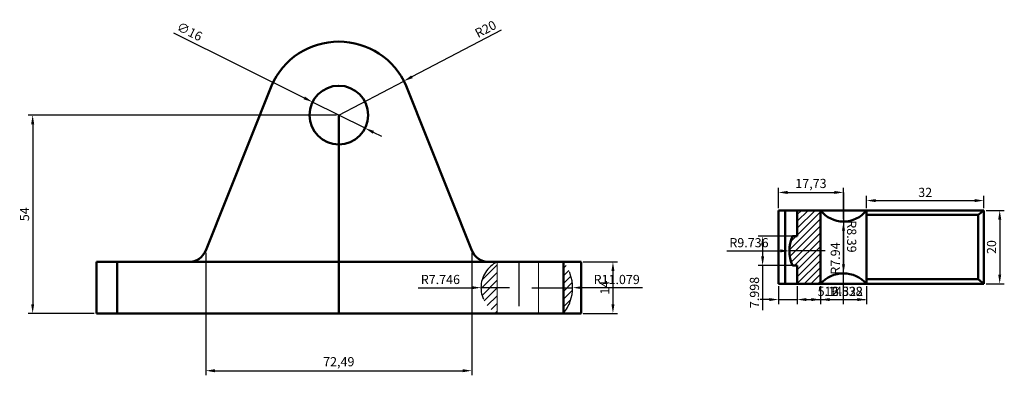
# Model space of a CAD drawing. Units: millimetres. Extents: x 1132 to 1696, y 1793 to 2376.
# Tile 2 of 4: x 1132 to 1400, y 1996 to 2093. Entities that reach past the tile are written whole.
import ezdxf

# ---------------------------------------------------------------- set-up
doc = ezdxf.new("R2010")
doc.units = ezdxf.units.MM
doc.linetypes.add('ACAD_ISO03W100', pattern=[30, 12, -18])
doc.linetypes.add('CENTER2', pattern=[28.575, 19.05, -3.175, 3.175, -3.175])
for name, color, linetype, lineweight in [('M-CNTR', 1, 'CENTER2', 18), ('M-DIMS', 2, 'Continuous', 25), ('M-HATC', 8, 'Continuous', 18), ('M-HIDN', 3, 'ACAD_ISO03W100', 25), ('M-OUTL', 7, 'Continuous', 50)]:
    doc.layers.add(name, color=color, linetype=linetype, lineweight=lineweight)
doc.styles.get("Standard").update_dxf_attribs({"font": 'arial.ttf'})
doc.dimstyles.new('ISO-25', dxfattribs={"dimtxt": 2.5, "dimasz": 2.5, "dimexe": 1.25, "dimexo": 0.625, "dimtad": 1, "dimtxsty": 'Standard', "dimcen": 2.5, "dimadec": 0, "dimazin": 0, "dimtfac": 1, "dimtmove": 0, "dimatfit": 3, "dimfxl": 1, "dimarcsym": 0})

# ---------------------------------------------------------------- blocks, each defined once
blk = doc.blocks.new('*D10')
at = {"layer": 'Defpoints', "color": 0, "transparency": 16777216}
for p in [(1182.57, 2029.81), (1255.05, 2029.81), (1255.05, 1997.05)]:
    blk.add_point(p, dxfattribs=at)
at = {"layer": 'M-DIMS', "color": 0, "lineweight": -2, "transparency": 16777216}
for p, q in [((1182.57, 2029.18), (1182.57, 1995.8)), ((1255.05, 2029.18), (1255.05, 1995.8)), ((1185.07, 1997.05), (1252.55, 1997.05))]:
    blk.add_line(p, q, dxfattribs=at)
at = {"layer": 'M-DIMS', "color": 0, "transparency": 16777216}
for points in [[(1185.07, 1997.47), (1185.07, 1996.63), (1182.57, 1997.05)], [(1252.55, 1997.47), (1252.55, 1996.63), (1255.05, 1997.05)]]:
    blk.add_solid(points, dxfattribs=at)
at = {"layer": 'M-DIMS', "color": 0, "transparency": 16777216, "insert": (1218.81, 1999.18), "char_height": 2.5, "attachment_point": 5}
blk.add_mtext('72,49', dxfattribs=at)
blk = doc.blocks.new('*D11')
at = {"layer": 'Defpoints', "color": 0, "transparency": 16777216}
for p in [(1284.81, 2026.66), (1284.81, 2012.66), (1293.51, 2012.66)]:
    blk.add_point(p, dxfattribs=at)
at = {"layer": 'M-DIMS', "color": 0, "lineweight": -2, "transparency": 16777216}
for p, q in [((1285.43, 2026.66), (1294.76, 2026.66)), ((1293.51, 2024.16), (1293.51, 2015.16)), ((1285.43, 2012.66), (1294.76, 2012.66))]:
    blk.add_line(p, q, dxfattribs=at)
at = {"layer": 'M-DIMS', "color": 0, "transparency": 16777216}
for points in [[(1293.09, 2024.16), (1293.93, 2024.16), (1293.51, 2026.66)], [(1293.09, 2015.16), (1293.93, 2015.16), (1293.51, 2012.66)]]:
    blk.add_solid(points, dxfattribs=at)
at = {"layer": 'M-DIMS', "color": 0, "transparency": 16777216, "insert": (1291.63, 2019.66), "char_height": 2.5, "attachment_point": 5, "rotation": 90}
blk.add_mtext('14', dxfattribs=at)
blk = doc.blocks.new('*D12')
at = {"layer": 'Defpoints', "color": 0, "transparency": 16777216}
for p in [(1218.81, 2066.66), (1135.4, 2012.66), (1152.81, 2012.66)]:
    blk.add_point(p, dxfattribs=at)
at = {"layer": 'M-DIMS', "color": 0, "lineweight": -2, "transparency": 16777216}
for p, q in [((1218.18, 2066.66), (1134.15, 2066.66)), ((1135.4, 2064.16), (1135.4, 2015.16)), ((1152.18, 2012.66), (1134.15, 2012.66))]:
    blk.add_line(p, q, dxfattribs=at)
at = {"layer": 'M-DIMS', "color": 0, "transparency": 16777216}
for points in [[(1134.98, 2064.16), (1135.82, 2064.16), (1135.4, 2066.66)], [(1134.98, 2015.16), (1135.82, 2015.16), (1135.4, 2012.66)]]:
    blk.add_solid(points, dxfattribs=at)
at = {"layer": 'M-DIMS', "color": 0, "transparency": 16777216, "insert": (1133.5, 2039.66), "char_height": 2.5, "attachment_point": 5, "rotation": 90}
blk.add_mtext('54', dxfattribs=at)
blk = doc.blocks.new('*D13')
at = {"layer": 'Defpoints', "color": 0, "transparency": 16777216}
for p in [(1236.53, 2075.93), (1218.81, 2066.66)]:
    blk.add_point(p, dxfattribs=at)
at = {"layer": 'M-DIMS', "color": 0, "lineweight": -2, "transparency": 16777216}
for p, q in [((1263.04, 2089.79), (1238.75, 2077.09)), ((1218.81, 2066.66), (1236.53, 2075.93))]:
    blk.add_line(p, q, dxfattribs=at)
at = {"layer": 'M-DIMS', "color": 0, "transparency": 16777216}
blk.add_solid([(1238.56, 2077.46), (1238.94, 2076.72), (1236.53, 2075.93)], dxfattribs=at)
at = {"layer": 'M-DIMS', "color": 0, "transparency": 16777216, "insert": (1258.96, 2089.81), "char_height": 2.5, "attachment_point": 5, "rotation": 27.6056}
blk.add_mtext('R20', dxfattribs=at)
blk = doc.blocks.new('*D14')
at = {"layer": 'Defpoints', "color": 0, "transparency": 16777216}
for p in [(1211.65, 2070.22), (1225.97, 2063.1)]:
    blk.add_point(p, dxfattribs=at)
at = {"layer": 'M-DIMS', "color": 0, "lineweight": -2, "transparency": 16777216}
for p, q in [((1173.76, 2089.05), (1209.41, 2071.34)), ((1225.97, 2063.1), (1211.65, 2070.22)), ((1228.21, 2061.99), (1230.45, 2060.88))]:
    blk.add_line(p, q, dxfattribs=at)
at = {"layer": 'M-DIMS', "color": 0, "transparency": 16777216}
for points in [[(1209.59, 2071.71), (1209.22, 2070.96), (1211.65, 2070.22)], [(1228.4, 2062.37), (1228.03, 2061.62), (1225.97, 2063.1)]]:
    blk.add_solid(points, dxfattribs=at)
at = {"layer": 'M-DIMS', "color": 0, "transparency": 16777216, "insert": (1178.02, 2089.13), "char_height": 2.5, "attachment_point": 5, "rotation": 333.5798}
blk.add_mtext('∅16', dxfattribs=at)
blk = doc.blocks.new('*D33')
at = {"layer": 'Defpoints', "color": 0, "transparency": 16777216}
for p in [(1394.59, 2043.38), (1362.59, 2040.72), (1394.59, 2040.72)]:
    blk.add_point(p, dxfattribs=at)
at = {"layer": 'M-DIMS', "color": 0, "lineweight": -2, "transparency": 16777216}
for p, q in [((1362.59, 2041.35), (1362.59, 2044.63)), ((1394.59, 2041.35), (1394.59, 2044.63)), ((1365.09, 2043.38), (1392.09, 2043.38))]:
    blk.add_line(p, q, dxfattribs=at)
at = {"layer": 'M-DIMS', "color": 0, "transparency": 16777216}
for points in [[(1365.09, 2043.79), (1365.09, 2042.96), (1362.59, 2043.38)], [(1392.09, 2043.79), (1392.09, 2042.96), (1394.59, 2043.38)]]:
    blk.add_solid(points, dxfattribs=at)
at = {"layer": 'M-DIMS', "color": 0, "transparency": 16777216, "insert": (1378.59, 2045.28), "char_height": 2.5, "attachment_point": 5}
blk.add_mtext('32', dxfattribs=at)
blk = doc.blocks.new('*D34')
at = {"layer": 'Defpoints', "color": 0, "transparency": 16777216}
for p in [(1356.33, 2045.6), (1338.59, 2040.72), (1356.33, 2037.65)]:
    blk.add_point(p, dxfattribs=at)
at = {"layer": 'M-DIMS', "color": 0, "lineweight": -2, "transparency": 16777216}
for p, q in [((1338.59, 2041.35), (1338.59, 2046.85)), ((1341.09, 2045.6), (1353.83, 2045.6)), ((1356.33, 2038.28), (1356.33, 2046.85))]:
    blk.add_line(p, q, dxfattribs=at)
at = {"layer": 'M-DIMS', "color": 0, "transparency": 16777216}
for points in [[(1341.09, 2046.01), (1341.09, 2045.18), (1338.59, 2045.6)], [(1353.83, 2046.01), (1353.83, 2045.18), (1356.33, 2045.6)]]:
    blk.add_solid(points, dxfattribs=at)
at = {"layer": 'M-DIMS', "color": 0, "transparency": 16777216, "insert": (1347.46, 2047.72), "char_height": 2.5, "attachment_point": 5}
blk.add_mtext('17,73', dxfattribs=at)
blk = doc.blocks.new('*D41')
at = {"layer": 'Defpoints', "color": 0, "transparency": 16777216}
for p in [(1394.59, 2040.72), (1394.59, 2020.72), (1398.89, 2020.72)]:
    blk.add_point(p, dxfattribs=at)
at = {"layer": 'M-DIMS', "color": 0, "lineweight": -2, "transparency": 16777216}
for p, q in [((1395.22, 2040.72), (1400.14, 2040.72)), ((1398.89, 2038.22), (1398.89, 2023.22)), ((1395.22, 2020.72), (1400.14, 2020.72))]:
    blk.add_line(p, q, dxfattribs=at)
at = {"layer": 'M-DIMS', "color": 0, "transparency": 16777216}
for points in [[(1398.48, 2038.22), (1399.31, 2038.22), (1398.89, 2040.72)], [(1398.48, 2023.22), (1399.31, 2023.22), (1398.89, 2020.72)]]:
    blk.add_solid(points, dxfattribs=at)
at = {"layer": 'M-DIMS', "color": 0, "transparency": 16777216, "insert": (1396.99, 2030.72), "char_height": 2.5, "attachment_point": 5, "rotation": 90}
blk.add_mtext('20', dxfattribs=at)
blk = doc.blocks.new('*D42')
at = {"layer": 'Defpoints', "color": 0, "transparency": 16777216}
for p in [(1338.59, 2020.72), (1343.73, 2020.72), (1343.73, 2016.42)]:
    blk.add_point(p, dxfattribs=at)
at = {"layer": 'M-DIMS', "color": 0, "lineweight": -2, "transparency": 16777216}
for p, q in [((1338.59, 2020.1), (1338.59, 2015.17)), ((1343.73, 2020.1), (1343.73, 2015.17)), ((1336.09, 2016.42), (1333.59, 2016.42)), ((1338.59, 2016.42), (1343.73, 2016.42)), ((1346.23, 2016.42), (1356.47, 2016.42))]:
    blk.add_line(p, q, dxfattribs=at)
at = {"layer": 'M-DIMS', "color": 0, "transparency": 16777216}
for points in [[(1336.09, 2016.84), (1336.09, 2016.01), (1338.59, 2016.42)], [(1346.23, 2016.84), (1346.23, 2016.01), (1343.73, 2016.42)]]:
    blk.add_solid(points, dxfattribs=at)
at = {"layer": 'M-DIMS', "color": 0, "transparency": 16777216, "insert": (1352.6, 2018.32), "char_height": 2.5, "attachment_point": 5}
blk.add_mtext('5.14', dxfattribs=at)
blk = doc.blocks.new('*D43')
at = {"layer": 'Defpoints', "color": 0, "transparency": 16777216}
for p in [(1343.73, 2020.72), (1350.06, 2020.72), (1350.06, 2016.42)]:
    blk.add_point(p, dxfattribs=at)
at = {"layer": 'M-DIMS', "color": 0, "lineweight": -2, "transparency": 16777216}
for p, q in [((1343.73, 2020.1), (1343.73, 2015.17)), ((1350.06, 2020.1), (1350.06, 2015.17)), ((1346.23, 2016.42), (1347.56, 2016.42)), ((1350.06, 2016.42), (1362.23, 2016.42))]:
    blk.add_line(p, q, dxfattribs=at)
at = {"layer": 'M-DIMS', "color": 0, "transparency": 16777216}
for points in [[(1346.23, 2016.84), (1346.23, 2016.01), (1343.73, 2016.42)], [(1347.56, 2016.84), (1347.56, 2016.01), (1350.06, 2016.42)]]:
    blk.add_solid(points, dxfattribs=at)
at = {"layer": 'M-DIMS', "color": 0, "transparency": 16777216, "insert": (1357.39, 2018.32), "char_height": 2.5, "attachment_point": 5}
blk.add_mtext('6.322', dxfattribs=at)
blk = doc.blocks.new('*D44')
at = {"layer": 'Defpoints', "color": 0, "transparency": 16777216}
for p in [(1350.06, 2020.72), (1362.59, 2020.72), (1362.59, 2016.42)]:
    blk.add_point(p, dxfattribs=at)
at = {"layer": 'M-DIMS', "color": 0, "lineweight": -2, "transparency": 16777216}
for p, q in [((1350.06, 2020.1), (1350.06, 2015.17)), ((1362.59, 2020.1), (1362.59, 2015.17)), ((1352.56, 2016.42), (1360.09, 2016.42))]:
    blk.add_line(p, q, dxfattribs=at)
at = {"layer": 'M-DIMS', "color": 0, "transparency": 16777216}
for points in [[(1352.56, 2016.84), (1352.56, 2016.01), (1350.06, 2016.42)], [(1360.09, 2016.84), (1360.09, 2016.01), (1362.59, 2016.42)]]:
    blk.add_solid(points, dxfattribs=at)
at = {"layer": 'M-DIMS', "color": 0, "transparency": 16777216, "insert": (1356.33, 2018.32), "char_height": 2.5, "attachment_point": 5}
blk.add_mtext('12.538', dxfattribs=at)
blk = doc.blocks.new('*D45')
at = {"layer": 'Defpoints', "color": 0, "transparency": 16777216}
for p in [(1343.73, 2033.68), (1334.29, 2025.68), (1343.73, 2025.68)]:
    blk.add_point(p, dxfattribs=at)
at = {"layer": 'M-DIMS', "color": 0, "lineweight": -2, "transparency": 16777216}
for p, q in [((1343.11, 2033.68), (1333.04, 2033.68)), ((1334.29, 2031.18), (1334.29, 2028.18)), ((1343.11, 2025.68), (1333.04, 2025.68)), ((1334.29, 2025.68), (1334.29, 2013.51))]:
    blk.add_line(p, q, dxfattribs=at)
at = {"layer": 'M-DIMS', "color": 0, "transparency": 16777216}
for points in [[(1333.88, 2031.18), (1334.71, 2031.18), (1334.29, 2033.68)], [(1333.88, 2028.18), (1334.71, 2028.18), (1334.29, 2025.68)]]:
    blk.add_solid(points, dxfattribs=at)
at = {"layer": 'M-DIMS', "color": 0, "transparency": 16777216, "insert": (1332.39, 2018.35), "char_height": 2.5, "attachment_point": 5, "rotation": 90}
blk.add_mtext('7.998', dxfattribs=at)
blk = doc.blocks.new('*D51')
at = {"layer": 'Defpoints', "color": 0, "transparency": 16777216}
for p in [(1356.33, 2023.54), (1356.33, 2015.15)]:
    blk.add_point(p, dxfattribs=at)
at = {"layer": 'M-DIMS', "color": 0, "lineweight": -2, "transparency": 16777216}
for p, q in [((1356.32, 2038.68), (1356.32, 2026.04)), ((1356.33, 2015.15), (1356.33, 2023.54))]:
    blk.add_line(p, q, dxfattribs=at)
at = {"layer": 'M-DIMS', "color": 0, "transparency": 16777216}
blk.add_solid([(1356.74, 2026.04), (1355.91, 2026.04), (1356.33, 2023.54)], dxfattribs=at)
at = {"layer": 'M-DIMS', "color": 0, "transparency": 16777216, "insert": (1358.23, 2033.61), "char_height": 2.5, "attachment_point": 5, "rotation": 270.003}
blk.add_mtext('R8.39', dxfattribs=at)
blk = doc.blocks.new('*D52')
at = {"layer": 'Defpoints', "color": 0, "transparency": 16777216}
for p in [(1356.33, 2045.6), (1356.33, 2037.65)]:
    blk.add_point(p, dxfattribs=at)
at = {"layer": 'M-DIMS', "color": 0, "lineweight": -2, "transparency": 16777216}
for p, q in [((1356.33, 2045.6), (1356.33, 2037.65)), ((1356.32, 2022.53), (1356.32, 2035.15))]:
    blk.add_line(p, q, dxfattribs=at)
at = {"layer": 'M-DIMS', "color": 0, "transparency": 16777216}
blk.add_solid([(1355.91, 2035.15), (1356.74, 2035.15), (1356.33, 2037.65)], dxfattribs=at)
at = {"layer": 'M-DIMS', "color": 0, "transparency": 16777216, "insert": (1354.42, 2027.59), "char_height": 2.5, "attachment_point": 5, "rotation": 89.9968}
blk.add_mtext('R7.94', dxfattribs=at)
blk = doc.blocks.new('*D53')
at = {"layer": 'Defpoints', "color": 0, "transparency": 16777216}
for p in [(1341.6, 2029.68), (1351.34, 2029.68)]:
    blk.add_point(p, dxfattribs=at)
at = {"layer": 'M-DIMS', "color": 0, "lineweight": -2, "transparency": 16777216}
for p, q in [((1324.53, 2029.68), (1339.1, 2029.68)), ((1351.34, 2029.68), (1341.6, 2029.68))]:
    blk.add_line(p, q, dxfattribs=at)
at = {"layer": 'M-DIMS', "color": 0, "transparency": 16777216}
blk.add_solid([(1339.1, 2030.1), (1339.1, 2029.27), (1341.6, 2029.68)], dxfattribs=at)
at = {"layer": 'M-DIMS', "color": 0, "transparency": 16777216, "insert": (1330.57, 2031.59), "char_height": 2.5, "attachment_point": 5, "rotation": 359.9988}
blk.add_mtext('R9.736', dxfattribs=at)
blk = doc.blocks.new('*D84')
at = {"layer": 'Defpoints', "color": 0, "transparency": 16777216}
for p in [(1271.44, 2019.66), (1282.52, 2019.66)]:
    blk.add_point(p, dxfattribs=at)
at = {"layer": 'M-DIMS', "color": 0, "lineweight": -2, "transparency": 16777216}
for p, q in [((1271.44, 2019.66), (1282.52, 2019.66)), ((1301.54, 2019.66), (1285.02, 2019.66))]:
    blk.add_line(p, q, dxfattribs=at)
at = {"layer": 'M-DIMS', "color": 0, "transparency": 16777216}
blk.add_solid([(1285.02, 2020.08), (1285.02, 2019.25), (1282.52, 2019.66)], dxfattribs=at)
at = {"layer": 'M-DIMS', "color": 0, "transparency": 16777216, "insert": (1294.53, 2021.57), "char_height": 2.5, "attachment_point": 5, "rotation": 359.9988}
blk.add_mtext('R11.079', dxfattribs=at)
blk = doc.blocks.new('*D85')
at = {"layer": 'Defpoints', "color": 0, "transparency": 16777216}
for p in [(1257.54, 2019.66), (1265.29, 2019.66)]:
    blk.add_point(p, dxfattribs=at)
at = {"layer": 'M-DIMS', "color": 0, "lineweight": -2, "transparency": 16777216}
for p, q in [((1240.46, 2019.66), (1255.04, 2019.66)), ((1265.29, 2019.66), (1257.54, 2019.66))]:
    blk.add_line(p, q, dxfattribs=at)
at = {"layer": 'M-DIMS', "color": 0, "transparency": 16777216}
blk.add_solid([(1255.04, 2020.08), (1255.04, 2019.25), (1257.54, 2019.66)], dxfattribs=at)
at = {"layer": 'M-DIMS', "color": 0, "transparency": 16777216, "insert": (1246.5, 2021.57), "char_height": 2.5, "attachment_point": 5, "rotation": 0.0018}
blk.add_mtext('R7.746', dxfattribs=at)

msp = doc.modelspace()

# ---------------------------------------------------------------- hatches: boundary and pattern name
at = {"layer": 'M-HATC'}
h = msp.add_hatch(dxfattribs=at)
h.set_pattern_fill('ANSI31', color=256, scale=0.42)
h.paths.add_polyline_path([(1350.0564, 2040.7218), (1343.7347, 2040.7218), (1343.7347, 2033.6829), (1342.4641, 2033.6829, 0.21485682), (1342.4641, 2025.6847), (1343.7347, 2025.6847), (1343.7347, 2020.7218), (1350.0564, 2020.7218)])
h = msp.add_hatch(dxfattribs=at)
h.set_pattern_fill('ANSI31', color=256, scale=0.47)
h.paths.add_polyline_path([(1261.968, 2026.6642, 0.6327158), (1261.968, 2012.6642)])
h.paths.add_polyline_path([(1280.0269, 2026.6642), (1280.0269, 2012.6642, 0.3559172)])

# ---------------------------------------------------------------- linework, layer by layer
at = {"layer": 'M-CNTR'}
for p, q in [((1261.968, 2026.6642), (1261.968, 2012.6642)), ((1273.1967, 2026.6642), (1273.1967, 2012.6642))]:
    msp.add_line(p, q, dxfattribs=at)
at = {"layer": 'M-HIDN'}
msp.add_line((1267.8741, 2026.6642), (1267.8741, 2012.6642), dxfattribs=at)
for centre, radius, start, end in [((1265.2852, 2019.6642), 7.7462, 115.355632, 244.644368), ((1271.4389, 2019.6642), 11.0795, 320.816962, 39.183038)]:
    msp.add_arc(centre, radius, start, end, dxfattribs=at)
at = {"layer": 'M-OUTL'}
for p, q in [((1200.4796, 2074.6642), (1182.5661, 2029.8098)), ((1237.1402, 2074.6642), (1255.0536, 2029.8098)), ((1218.8099, 2012.6642), (1218.8099, 2066.6642)), ((1394.5945, 2040.7218), (1338.5945, 2040.7218)), ((1338.5945, 2040.7218), (1338.5945, 2020.7218)), ((1340.478, 2040.7218), (1340.478, 2020.7218)), ((1343.7347, 2040.7218), (1343.7347, 2033.6829)), ((1350.0564, 2040.7218), (1350.0564, 2020.7218)), ((1362.5945, 2040.7218), (1362.5945, 2020.7218)), ((1393.0194, 2039.5194), (1362.5945, 2039.5194)), ((1393.0194, 2039.5194), (1394.5945, 2040.7218)), ((1393.0194, 2021.9378), (1393.0194, 2039.5194)), ((1394.5945, 2020.7218), (1394.5945, 2040.7218)), ((1342.4641, 2033.6829), (1343.7347, 2033.6829)), ((1152.8099, 2026.6642), (1152.8099, 2012.6642)), ((1177.9227, 2026.6642), (1152.8099, 2026.6642)), ((1158.4024, 2026.6642), (1158.4024, 2012.6642)), ((1177.9227, 2026.6642), (1256.3099, 2026.6642)), ((1218.8099, 2026.6642), (1256.3099, 2026.6642)), ((1256.3099, 2026.6642), (1261.968, 2026.6642)), ((1259.697, 2026.6642), (1284.8099, 2026.6642)), ((1280.0269, 2012.6642), (1280.0269, 2026.6642)), ((1284.8099, 2012.6642), (1284.8099, 2026.6642)), ((1343.7347, 2025.6847), (1342.4641, 2025.6847)), ((1343.7347, 2025.6847), (1343.7347, 2020.7218)), ((1338.5945, 2020.7218), (1394.5945, 2020.7218)), ((1362.5945, 2021.9378), (1393.0194, 2021.9378)), ((1393.0194, 2021.9378), (1394.5945, 2020.7218)), ((1152.8099, 2012.6642), (1284.8099, 2012.6642)), ((1218.8099, 2012.6642), (1181.3099, 2012.6642))]:
    msp.add_line(p, q, dxfattribs=at)
msp.add_circle((1218.8099, 2066.6642), 8, dxfattribs=at)
for centre, radius, start, end in [((1218.8099, 2066.6642), 20, 23.578178, 156.421822), ((1356.3254, 2045.5953), 7.9406, 217.86123, 322.13877), ((1351.3409, 2029.6838), 9.736, 155.747922, 204.252078), ((1177.9227, 2031.6642), 5, 270, 338.229779), ((1259.697, 2031.6642), 5, 201.770221, 270), ((1356.3254, 2015.145), 8.3906, 41.655372, 138.344628)]:
    msp.add_arc(centre, radius, start, end, dxfattribs=at)

# ---------------------------------------------------------------- dimensions: what is measured, and where the dimension line sits
at = {"layer": 'M-DIMS'}
dim = msp.add_radius_dim(center=(1218.8099, 2066.6642), mpoint=(1236.533, 2075.9319), dimstyle='ISO-25', override={"dimclrd": 0, "dimclre": 0, "dimclrt": 0}, dxfattribs=at)
dim.commit()
dim.dimension.update_dxf_attribs({"geometry": '*D13', "text_midpoint": (1259.8413, 2088.1201), "dimtype": 164})
dim = msp.add_diameter_dim_2p(p1=(1225.9743, 2063.1046), p2=(1211.6454, 2070.2238), dimstyle='ISO-25', override={"dimclrd": 0, "dimclre": 0, "dimclrt": 0}, dxfattribs=at)
dim.commit()
dim.dimension.update_dxf_attribs({"geometry": '*D14', "text_midpoint": (1177.142, 2087.3666), "dimtype": 163})
for base, p1, p2, override, picture, middle in [((1135.4003, 2012.6642), (1218.8099, 2066.6642), (1152.8099, 2012.6642), {"dimclrd": 0, "dimclre": 0, "dimclrt": 0}, '*D12', (1133.504, 2039.6642)), ((1398.8945, 2020.7218), (1394.5945, 2040.7218), (1394.5945, 2020.7218), {"dimdec": 0, "dimlfac": 1, "dimrnd": 0, "dimzin": 0, "dimdsep": 46, "dimlunit": 2}, '*D41', (1396.9931, 2030.7218)), ((1334.2945, 2025.6847), (1343.7347, 2033.6829), (1343.7347, 2025.6847), {"dimdec": 3, "dimlfac": 1, "dimrnd": 0, "dimzin": 0, "dimdsep": 46, "dimlunit": 2}, '*D45', (1332.3931, 2018.3493)), ((1293.5095, 2012.6642), (1284.8099, 2026.6642), (1284.8099, 2012.6642), {"dimclrd": 0, "dimclre": 0, "dimclrt": 0}, '*D11', (1291.6293, 2019.6642))]:
    dim = msp.add_linear_dim(base=base, p1=p1, p2=p2, angle=90, dimstyle='ISO-25', override=override, dxfattribs=at)
    dim.commit()
    dim.dimension.update_dxf_attribs({"geometry": picture, "text_midpoint": middle})
for base, p1, p2, override, picture, middle in [((1356.3254, 2045.5953), (1338.5945, 2040.7218), (1356.3254, 2037.6548), {"dimclrd": 0, "dimclre": 0, "dimclrt": 0}, '*D34', (1347.46, 2047.7227)), ((1394.5945, 2043.3763), (1362.5945, 2040.7218), (1394.5945, 2040.7218), {"dimclrd": 0, "dimclre": 0, "dimclrt": 0}, '*D33', (1378.5945, 2045.2786)), ((1255.0536, 1997.0507), (1182.5661, 2029.8098), (1255.0536, 2029.8098), {"dimclrd": 0, "dimclre": 0, "dimclrt": 0}, '*D10', (1218.8099, 1999.1781)), ((1343.7347, 2016.4218), (1338.5945, 2020.7218), (1343.7347, 2020.7218), {"dimdec": 2, "dimlfac": 1, "dimrnd": 0, "dimzin": 0, "dimdsep": 46, "dimlunit": 2}, '*D42', (1352.6015, 2018.3232)), ((1350.0564, 2016.4218), (1343.7347, 2020.7218), (1350.0564, 2020.7218), {"dimdec": 3, "dimlfac": 1, "dimrnd": 0, "dimzin": 0, "dimdsep": 46, "dimlunit": 2}, '*D43', (1357.3935, 2018.3241)), ((1362.5945, 2016.4218), (1350.0564, 2020.7218), (1362.5945, 2020.7218), {"dimdec": 3, "dimlfac": 1, "dimrnd": 0, "dimzin": 0, "dimdsep": 46, "dimlunit": 2}, '*D44', (1356.3254, 2018.3241))]:
    dim = msp.add_linear_dim(base=base, p1=p1, p2=p2, dimstyle='ISO-25', override=override, dxfattribs=at)
    dim.commit()
    dim.dimension.update_dxf_attribs({"geometry": picture, "text_midpoint": middle})
for center, mpoint, override, picture, middle in [((1356.3254, 2045.5953), (1356.325, 2037.6548), {"dimdec": 2, "dimlfac": 1, "dimrnd": 0, "dimzin": 0, "dimdsep": 46, "dimlunit": 2}, '*D52', (1354.423, 2027.5918)), ((1356.3254, 2015.145), (1356.325, 2023.5356), {"dimdec": 2, "dimlfac": 1, "dimrnd": 0, "dimzin": 0, "dimdsep": 46, "dimlunit": 2}, '*D51', (1358.2267, 2033.6065)), ((1351.3409, 2029.6838), (1341.6049, 2029.684), {"dimdec": 3, "dimlfac": 1, "dimrnd": 0, "dimzin": 0, "dimdsep": 46, "dimlunit": 2}, '*D53', (1330.5664, 2031.5865)), ((1265.2852, 2019.6642), (1257.539, 2019.664), {"dimdec": 3, "dimlfac": 1, "dimrnd": 0, "dimzin": 0, "dimdsep": 46, "dimlunit": 2}, '*D85', (1246.5004, 2021.5651)), ((1271.4389, 2019.6642), (1282.5183, 2019.664), {"dimdec": 3, "dimlfac": 1, "dimrnd": 0, "dimzin": 0, "dimdsep": 46, "dimlunit": 2}, '*D84', (1294.5315, 2021.5652))]:
    dim = msp.add_radius_dim(center=center, mpoint=mpoint, dimstyle='ISO-25', override=override, dxfattribs=at)
    dim.commit()
    dim.dimension.update_dxf_attribs({"geometry": picture, "text_midpoint": middle})

doc.saveas('drawing.dxf')
